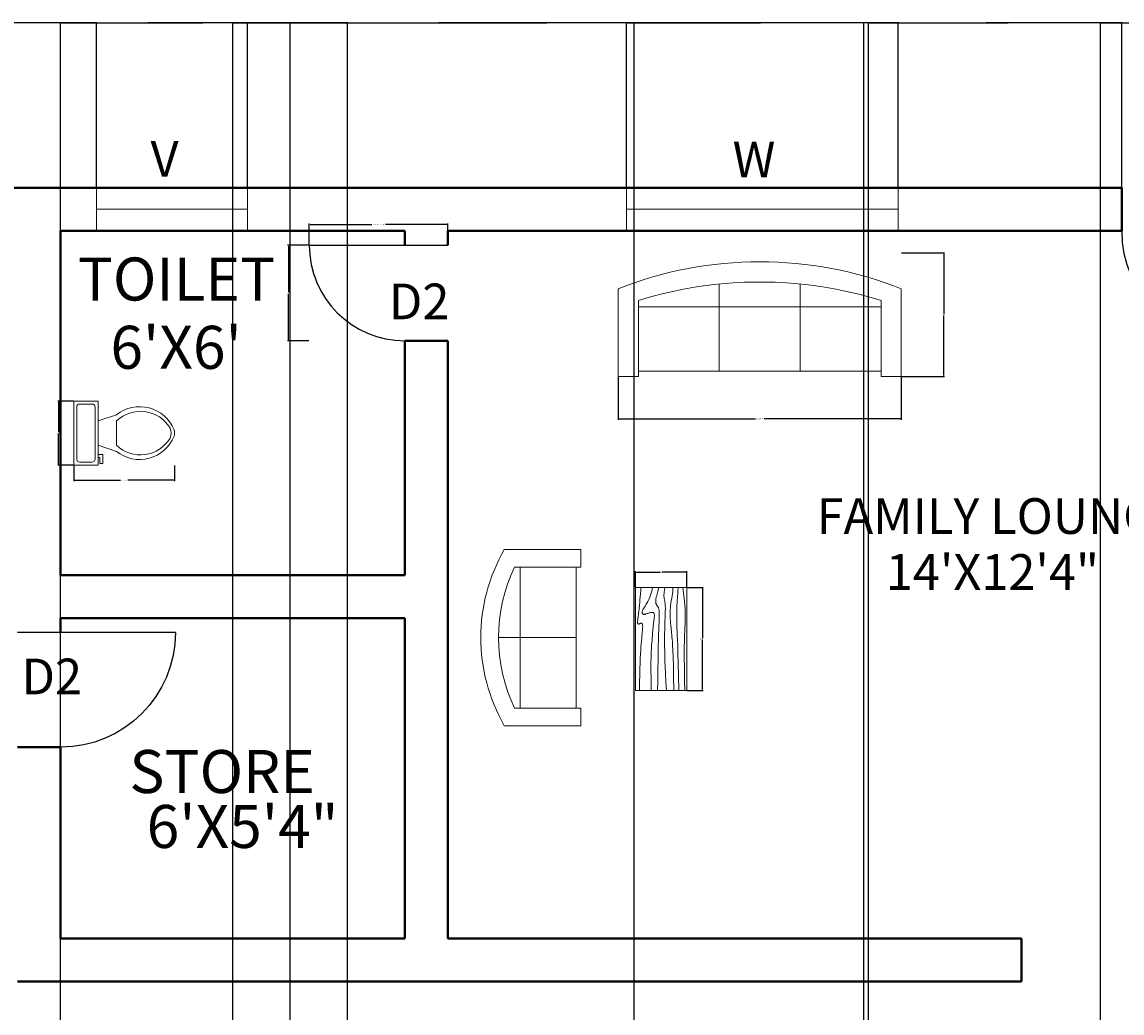
# Model space of a CAD drawing. Units: feet. Extents: x 2032 to 2763, y 1402 to 2145.
# Tile 5 of 6: x 2285 to 2515, y 1938 to 2145. Entities that reach past the tile are written whole.
import ezdxf

# ---------------------------------------------------------------- set-up
doc = ezdxf.new("R2010")
doc.units = ezdxf.units.FT
for name, color, linetype, lineweight in [('A-ANNO-DIMS', 2, 'Continuous', 18), ('A-ANNO-TEXT', 7, 'Continuous', 18), ('A-AREA-IDEN', 7, 'Continuous', 25), ('A-DOOR', 3, 'Continuous', 25), ('A-FLOR-FIXT', 8, 'Continuous', 18), ('A-FURN', 8, 'Continuous', 18), ('A-GLAZ', 4, 'Continuous', 18), ('A-WALL', 7, 'Continuous', 40)]:
    doc.layers.add(name, color=color, linetype=linetype, lineweight=lineweight)
doc.styles.get("Standard").update_dxf_attribs({"font": 'arial.ttf'})
doc.dimstyles.get("Standard").update_dxf_attribs({"dimtxt": 0.18, "dimasz": 0.18, "dimexe": 0.18, "dimexo": 0.0625, "dimgap": 0.09, "dimtad": 0, "dimtih": 1, "dimtoh": 1, "dimdec": 4, "dimzin": 0, "dimdsep": 46, "dimtxsty": 'Standard', "dimcen": 0.09, "dimadec": 0, "dimazin": 0, "dimtfac": 1, "dimtdec": 4, "dimtofl": 0, "dimtmove": 0, "dimatfit": 3, "dimfxl": 1, "dimtolj": 1, "dimtzin": 0, "dimarcsym": 0})

# ---------------------------------------------------------------- blocks, each defined once
blk = doc.blocks.new('Toilet - top')
for p, q in [((9.5, -6), (9.5, -2)), ((-10, -8.5), (-8, -8.5)), ((-10, -9.5), (-10, -8.5)), ((-7, -9.5), (-10, -9.5)), ((-8, -8.5), (-8, -8)), ((-7, -8), (-7, -9.5)), ((-4, -8), (-6, -14)), ((4, -8), (6, -14)), ((4, -14), (-4, -14))]:
    blk.add_line(p, q)
blk.add_lwpolyline([(10.5, -8), (10.5, 0), (-10.5, 0), (-10.5, -8)], close=True)
for points in [[(-9.5, -2), (-9.5, -6)], [(8.5, -1), (-8.5, -1)], [(-8.5, -7), (8.5, -7)]]:
    blk.add_lwpolyline(points)
for centre, radius, start, end in [((-8.62, -1.88), 0.884, 81.8699, 188.1301), ((8.62, -1.88), 0.884, 351.8699, 98.1301), ((-8.62, -6.12), 0.884, 171.8699, 278.1301), ((8.62, -6.12), 0.884, 261.8699, 8.1301), ((3.52, -21.58), 12.17, 141.4691, 247.9714), ((4.2, -21.82), 11.33, 136.3677, 238.9468), ((-3.52, -21.58), 12.17, 292.0284, 38.5307), ((-4.2, -21.82), 11.33, 301.053, 43.6321), ((0, -27.88), 4, 245.7318, 294.2682), ((0, -29), 4, 254.8605, 285.1395)]:
    blk.add_arc(centre, radius, start, end)
blk = doc.blocks.new('Sofa - Roundback 7 ft.')
for p, q in [((-12.00002, -32.4421), (-12.00003, -6.5971)), ((11.99997, -32.4421), (11.99998, -6.5971)), ((-36.000027, -34), (-36.000027, -11.4696)), ((35.99998, -34), (35.99998, -11.4696)), ((-35.999844, -13.3819), (35.9998, -13.3819)), ((-36.000027, -32.4421), (35.99998, -32.4421))]:
    blk.add_line(p, q)
for points in [[(-36.000027, -34), (-42.000027, -34), (-42.000027, -8)], [(41.99998, -8), (41.99998, -34), (35.99998, -34)]]:
    blk.add_lwpolyline(points)
for centre, radius, start, end in [((0, -114.25), 114.25, 68.43141, 111.5686), ((-0.00001, -127.1968), 121.1968, 72.72033, 107.2797)]:
    blk.add_arc(centre, radius, start, end)
blk = doc.blocks.new('Sofa - Roundback Loveseat 5 ft.')
for p, q in [((0, -32.44198), (0, -5.99998)), ((-24, -33.99998), (-24, -11.46958)), ((-23.9998, -13.38178), (23.99986, -13.38178)), ((24.00004, -33.99998), (24.00004, -11.46958)), ((-24, -32.44198), (24.00004, -32.44198))]:
    blk.add_line(p, q)
for points in [[(-24, -33.99998), (-30, -33.99998), (-30, -7.99998)], [(30.00004, -7.99998), (30.00004, -33.99998), (24.00004, -33.99998)]]:
    blk.add_lwpolyline(points)
for centre, radius, start, end in [((0, -60.24998), 60.24998, 60.13715, 119.8628), ((0, -61.38438), 55.38444, 64.32083, 115.6792)]:
    blk.add_arc(centre, radius, start, end)
blk = doc.blocks.new('Table - Rectangular Woodgrain 60 x 30 in.')
for p, q in [((0, 0), (0, -30)), ((60, 0), (0, 0)), ((60, -30), (60, 0)), ((0, -30), (60, -30))]:
    blk.add_line(p, q)
for points in [[(0, -2.4), (4.8155, -2.418), (9.0302, -2.4688), (12.709, -2.5477), (15.9167, -2.65), (18.7181, -2.7711), (21.1781, -2.9063), (23.3616, -3.0508), (25.3333, -3.2), (27.1477, -3.3495), (28.8172, -3.4958), (30.3437, -3.636), (31.7291, -3.7667), (32.9756, -3.8849), (34.0849, -3.9875), (35.059, -4.0714), (35.9, -4.1334), (36.6114, -4.1711), (37.2041, -4.1854), (37.6906, -4.1779), (38.0833, -4.15), (38.3948, -4.1034), (38.6375, -4.0396), (38.8239, -3.9602), (38.9666, -3.8667), (39.0764, -3.7608), (39.1573, -3.6448), (39.2116, -3.521), (39.2416, -3.3917), (39.2498, -3.2593), (39.2385, -3.1261), (39.21, -2.9944), (39.1666, -2.8667), (39.111, -2.7447), (39.0468, -2.6281), (38.978, -2.5163), (38.9083, -2.4083), (38.8418, -2.3035), (38.7823, -2.201), (38.7337, -2.1001), (38.7, -2), (38.6844, -1.9003), (38.6875, -1.8021), (38.7094, -1.707), (38.75, -1.6167), (38.8094, -1.5326), (38.8875, -1.4563), (38.9844, -1.3893), (39.1, -1.3333), (39.2351, -1.2896), (39.3937, -1.2583), (39.5804, -1.2396), (39.8, -1.2333), (40.057, -1.2396), (40.3562, -1.2583), (40.7023, -1.2896), (41.1, -1.3333), (41.5547, -1.3895), (42.0755, -1.4573), (42.6721, -1.5361), (43.3542, -1.625), (44.1316, -1.7233), (45.014, -1.8302), (46.0114, -1.9449), (47.1333, -2.0667), (48.3862, -2.1947), (49.7625, -2.3281), (51.2513, -2.4663), (52.8416, -2.6083), (54.5226, -2.7535), (56.2833, -2.9011), (58.1127, -3.0501), (60, -3.2)], [(0, -9.2), (6.5759, -9.0858), (11.9385, -9.0365), (16.2527, -9.0418), (19.6833, -9.0917), (22.3952, -9.1759), (24.5531, -9.2844), (26.322, -9.4069), (27.8666, -9.5333), (29.3241, -9.6553), (30.7203, -9.7719), (32.0532, -9.8837), (33.3208, -9.9917), (34.5213, -10.0965), (35.6526, -10.199), (36.7128, -10.2999), (37.7, -10.4), (38.6129, -10.4996), (39.4531, -10.5969), (40.223, -10.6895), (40.925, -10.775), (41.5613, -10.8512), (42.1344, -10.9156), (42.6465, -10.966), (43.1, -11), (43.4976, -11.0158), (43.8437, -11.0136), (44.143, -10.9942), (44.4, -10.9583), (44.6195, -10.9069), (44.8062, -10.8406), (44.9648, -10.7603), (45.1, -10.6667), (45.2155, -10.5598), (45.3114, -10.4365), (45.3871, -10.2929), (45.4416, -10.125), (45.4743, -9.929), (45.4844, -9.7011), (45.4709, -9.4371), (45.4333, -9.1333), (45.3716, -8.7883), (45.2896, -8.4104), (45.1919, -8.0107), (45.0833, -7.6), (44.9685, -7.1893), (44.8521, -6.7896), (44.7388, -6.4117), (44.6333, -6.0667), (44.54, -5.7628), (44.4614, -5.4979), (44.4001, -5.2675), (44.3583, -5.0667), (44.3384, -4.8909), (44.3427, -4.7354), (44.3736, -4.5956), (44.4333, -4.4667), (44.5236, -4.3453), (44.6427, -4.2333), (44.7884, -4.1339), (44.9583, -4.05), (45.1501, -3.9849), (45.3614, -3.9417), (45.59, -3.9234), (45.8333, -3.9333), (46.0915, -3.9749), (46.3734, -4.0531), (46.6906, -4.1736), (47.0542, -4.3417), (47.4756, -4.5629), (47.9661, -4.8427), (48.5372, -5.1866), (49.2, -5.6), (49.9676, -6.0844), (50.8594, -6.625), (51.8965, -7.2031), (53.1, -7.8), (54.491, -8.3969), (56.0906, -8.975), (57.9199, -9.5156), (60, -10)], [(0, -12.8), (5.1847, -12.9322), (9.6213, -13.0323), (13.3963, -13.1059), (16.5958, -13.1583), (19.3063, -13.1952), (21.614, -13.2219), (23.6054, -13.2439), (25.3666, -13.2667), (26.9728, -13.2947), (28.4531, -13.3281), (29.8256, -13.3663), (31.1083, -13.4083), (32.3191, -13.4535), (33.476, -13.501), (34.597, -13.5501), (35.7, -13.6), (36.7984, -13.6497), (37.8875, -13.6979), (38.9578, -13.743), (40, -13.7833), (41.0047, -13.8174), (41.9625, -13.8438), (42.864, -13.8607), (43.7, -13.8667), (44.4631, -13.8604), (45.1552, -13.8417), (45.7801, -13.8104), (46.3416, -13.7667), (46.8439, -13.7104), (47.2906, -13.6417), (47.6858, -13.5604), (48.0333, -13.4667), (48.3375, -13.3608), (48.6042, -13.2448), (48.8396, -13.121), (49.05, -12.9917), (49.2417, -12.8593), (49.4208, -12.7261), (49.5937, -12.5944), (49.7667, -12.4667), (49.9452, -12.3451), (50.1323, -12.2313), (50.3303, -12.1268), (50.5416, -12.0333), (50.7686, -11.9524), (51.0135, -11.8854), (51.2788, -11.8341), (51.5666, -11.8), (51.8785, -11.7843), (52.2116, -11.7865), (52.562, -11.8059), (52.926, -11.8417), (53.2998, -11.8931), (53.6795, -11.9594), (54.0614, -12.0397), (54.4416, -12.1333), (54.8223, -12.2401), (55.2293, -12.3625), (55.6942, -12.5037), (56.2489, -12.6667), (56.9251, -12.8547), (57.7545, -13.0708), (58.7689, -13.3182), (60, -13.6)], [(0, -18), (5.124, -17.7273), (9.6609, -17.5057), (13.6705, -17.3303), (17.2125, -17.1958), (20.3467, -17.0973), (23.1328, -17.0297), (25.6307, -16.9878), (27.9, -16.9667), (29.9928, -16.9617), (31.9302, -16.9703), (33.7254, -16.9907), (35.3917, -17.0208), (36.9423, -17.0588), (38.3906, -17.1026), (39.7499, -17.1503), (41.0333, -17.2), (42.2519, -17.2496), (43.4073, -17.2969), (44.4986, -17.3395), (45.525, -17.375), (46.4858, -17.4012), (47.3802, -17.4156), (48.2074, -17.416), (48.9667, -17.4), (49.6583, -17.3662), (50.2872, -17.3167), (50.8595, -17.2547), (51.3812, -17.1833), (51.8584, -17.1057), (52.2971, -17.025), (52.7034, -16.9443), (53.0833, -16.8667), (53.443, -16.7951), (53.789, -16.7313), (54.128, -16.6768), (54.4666, -16.6334), (54.8115, -16.6024), (55.1693, -16.5854), (55.5465, -16.5841), (55.95, -16.6), (56.3828, -16.6337), (56.8346, -16.6823), (57.2915, -16.7418), (57.7396, -16.8084), (58.165, -16.878), (58.5539, -16.9469), (58.8924, -17.0111), (59.1666, -17.0667), (59.3679, -17.1107), (59.5078, -17.1438), (59.6032, -17.1675), (59.6708, -17.1833), (59.7275, -17.193), (59.7901, -17.1979), (59.8753, -17.1998), (60, -17.2)], [(0, -22.4), (8.0098, -22.2501), (14.4094, -22.1011), (19.4168, -21.9535), (23.25, -21.8083), (26.1269, -21.6663), (28.2656, -21.5281), (29.884, -21.3947), (31.2, -21.2667), (32.3967, -21.1448), (33.5172, -21.0292), (34.5697, -20.9198), (35.5625, -20.8167), (36.5037, -20.7198), (37.4015, -20.6292), (38.2642, -20.5448), (39.1, -20.4667), (39.9164, -20.3951), (40.7187, -20.3313), (41.5117, -20.2768), (42.3, -20.2333), (43.0883, -20.2024), (43.8812, -20.1854), (44.6836, -20.1841), (45.5, -20.2), (46.3328, -20.234), (47.1747, -20.2844), (48.0163, -20.3488), (48.8479, -20.425), (49.66, -20.5106), (50.4429, -20.6031), (51.1872, -20.7004), (51.8833, -20.8), (52.5246, -20.8999), (53.1166, -20.9995), (53.6681, -21.0983), (54.1875, -21.1958), (54.6834, -21.2919), (55.1646, -21.3859), (55.6394, -21.4777), (56.1167, -21.5667), (56.6028, -21.6515), (57.0961, -21.7266), (57.5929, -21.7852), (58.0896, -21.8208), (58.5823, -21.8268), (59.0674, -21.7964), (59.5412, -21.723), (60, -21.6)], [(0, -25.2), (8.6355, -25.0504), (15.7026, -24.9031), (21.4049, -24.7606), (25.9458, -24.625), (29.529, -24.4988), (32.3578, -24.3844), (34.6359, -24.284), (36.5667, -24.2), (38.3213, -24.1341), (39.9417, -24.0854), (41.437, -24.0523), (42.8167, -24.0333), (44.0901, -24.0268), (45.2667, -24.0313), (46.3557, -24.0451), (47.3667, -24.0667), (48.309, -24.0947), (49.1928, -24.1287), (50.0284, -24.168), (50.826, -24.2125), (51.5959, -24.2617), (52.3483, -24.3151), (53.0935, -24.3725), (53.8417, -24.4334), (54.6009, -24.497), (55.3699, -24.561), (56.1454, -24.6226), (56.9239, -24.6792), (57.7021, -24.7279), (58.4764, -24.7662), (59.2435, -24.7911), (60, -24.8)], [(0, -28.8), (5.6867, -28.6681), (10.45, -28.5698), (14.407, -28.5012), (17.675, -28.4584), (20.3711, -28.4374), (22.6125, -28.4344), (24.5164, -28.4455), (26.2, -28.4667), (27.762, -28.4947), (29.2276, -28.5281), (30.6033, -28.5663), (31.8958, -28.6084), (33.1118, -28.6535), (34.2578, -28.7011), (35.3405, -28.7501), (36.3666, -28.8), (37.3443, -28.8497), (38.288, -28.8974), (39.2137, -28.9412), (40.1375, -28.9792), (41.0753, -29.0093), (42.0432, -29.0297), (43.0572, -29.0384), (44.1333, -29.0333), (45.2936, -29.0114), (46.5843, -28.9641), (48.0579, -28.8816), (49.7666, -28.7542), (51.7629, -28.5721), (54.0989, -28.3255), (56.8272, -28.0048), (60, -27.6)]]:
    blk.add_lwpolyline(points)
blk = doc.blocks.new('DOOR-SWING-24')
blk.add_line((33, 0), (0, 0))
blk.add_arc((9, 0), 24, 0, 90)
blk = doc.blocks.new('DOOR-SWING-20')
blk.add_line((0, 20), (29, 20))
blk.add_arc((20, 20), 20, 180, 270)
blk = doc.blocks.new('*D13')
at = {"layer": 'A-ANNO-DIMS', "color": 0, "lineweight": -2, "transparency": 16777216}
for p, q in [((2296.05, 2052.54), (2296.05, 2049.26)), ((2317.16, 2052.54), (2317.16, 2049.26)), ((2296.23, 2049.44), (2305.83, 2049.44)), ((2316.98, 2049.44), (2307.38, 2049.44))]:
    blk.add_line(p, q, dxfattribs=at)
at = {"layer": 'A-ANNO-DIMS', "color": 0, "transparency": 16777216}
for points in [[(2296.23, 2049.47), (2296.23, 2049.41), (2296.05, 2049.44)], [(2316.98, 2049.47), (2316.98, 2049.41), (2317.16, 2049.44)]]:
    blk.add_solid(points, dxfattribs=at)
at = {"layer": 'Defpoints', "color": 0, "transparency": 16777216}
for p in [(2296.05, 2052.6), (2317.16, 2052.6), (2296.05, 2049.44)]:
    blk.add_point(p, dxfattribs=at)
at = {"layer": 'A-ANNO-DIMS', "color": 0, "transparency": 16777216, "insert": (2306.61, 2049.44), "char_height": 0.18, "attachment_point": 5}
blk.add_mtext('\\A1;WC 21 TYP.', dxfattribs=at)
blk = doc.blocks.new('*D14')
at = {"layer": 'A-ANNO-DIMS', "color": 0, "lineweight": -2, "transparency": 16777216}
for p, q in [((2295.99, 2066.02), (2292.7, 2066.02)), ((2292.88, 2065.84), (2292.88, 2059.49)), ((2292.88, 2052.78), (2292.88, 2059.13)), ((2295.99, 2052.6), (2292.7, 2052.6))]:
    blk.add_line(p, q, dxfattribs=at)
at = {"layer": 'A-ANNO-DIMS', "color": 0, "transparency": 16777216}
for points in [[(2292.85, 2065.84), (2292.91, 2065.84), (2292.88, 2066.02)], [(2292.85, 2052.78), (2292.91, 2052.78), (2292.88, 2052.6)]]:
    blk.add_solid(points, dxfattribs=at)
at = {"layer": 'Defpoints', "color": 0, "transparency": 16777216}
for p in [(2292.88, 2066.02), (2296.05, 2066.02), (2296.05, 2052.6)]:
    blk.add_point(p, dxfattribs=at)
at = {"layer": 'A-ANNO-DIMS', "color": 0, "transparency": 16777216, "insert": (2292.88, 2059.31), "char_height": 0.18, "attachment_point": 5}
blk.add_mtext('\\A1;13 TYP.', dxfattribs=at)
blk = doc.blocks.new('*D17')
at = {"layer": 'A-ANNO-DIMS', "color": 0, "lineweight": -2, "transparency": 16777216}
for p, q in [((2409.94, 2071.12), (2409.94, 2062.12)), ((2469.15, 2071.12), (2469.15, 2062.12)), ((2410.12, 2062.3), (2438.64, 2062.3)), ((2468.97, 2062.3), (2440.45, 2062.3))]:
    blk.add_line(p, q, dxfattribs=at)
at = {"layer": 'A-ANNO-DIMS', "color": 0, "transparency": 16777216}
for points in [[(2410.12, 2062.33), (2410.12, 2062.27), (2409.94, 2062.3)], [(2468.97, 2062.33), (2468.97, 2062.27), (2469.15, 2062.3)]]:
    blk.add_solid(points, dxfattribs=at)
at = {"layer": 'Defpoints', "color": 0, "transparency": 16777216}
for p in [(2409.94, 2071.18), (2469.15, 2071.18), (2469.15, 2062.3)]:
    blk.add_point(p, dxfattribs=at)
at = {"layer": 'A-ANNO-DIMS', "color": 0, "transparency": 16777216, "insert": (2439.54, 2062.3), "char_height": 0.18, "attachment_point": 5}
blk.add_mtext('\\A1;SOFA 59 TYP.', dxfattribs=at)
blk = doc.blocks.new('*D18')
at = {"layer": 'A-ANNO-DIMS', "color": 0, "lineweight": -2, "transparency": 16777216}
for p, q in [((2469.21, 2097.02), (2478.21, 2097.02)), ((2478.03, 2096.84), (2478.03, 2084.28)), ((2478.03, 2071.36), (2478.03, 2083.92)), ((2469.21, 2071.18), (2478.21, 2071.18))]:
    blk.add_line(p, q, dxfattribs=at)
at = {"layer": 'A-ANNO-DIMS', "color": 0, "transparency": 16777216}
for points in [[(2478, 2096.84), (2478.06, 2096.84), (2478.03, 2097.02)], [(2478, 2071.36), (2478.06, 2071.36), (2478.03, 2071.18)]]:
    blk.add_solid(points, dxfattribs=at)
at = {"layer": 'Defpoints', "color": 0, "transparency": 16777216}
for p in [(2469.15, 2097.02), (2478.03, 2097.02), (2469.15, 2071.18)]:
    blk.add_point(p, dxfattribs=at)
at = {"layer": 'A-ANNO-DIMS', "color": 0, "transparency": 16777216, "insert": (2478.03, 2084.1), "char_height": 0.18, "attachment_point": 5}
blk.add_mtext('\\A1;26 TYP.', dxfattribs=at)
blk = doc.blocks.new('*D21')
at = {"layer": 'A-ANNO-DIMS', "color": 0, "lineweight": -2, "transparency": 16777216}
for p, q in [((2424.38, 2027.01), (2427.72, 2027.01)), ((2427.54, 2026.83), (2427.54, 2016.42)), ((2427.54, 2005.66), (2427.54, 2016.06)), ((2424.38, 2005.48), (2427.72, 2005.48))]:
    blk.add_line(p, q, dxfattribs=at)
at = {"layer": 'A-ANNO-DIMS', "color": 0, "transparency": 16777216}
for points in [[(2427.51, 2026.83), (2427.57, 2026.83), (2427.54, 2027.01)], [(2427.51, 2005.66), (2427.57, 2005.66), (2427.54, 2005.48)]]:
    blk.add_solid(points, dxfattribs=at)
at = {"layer": 'Defpoints', "color": 0, "transparency": 16777216}
for p in [(2424.31, 2027.01), (2427.54, 2027.01), (2424.31, 2005.48)]:
    blk.add_point(p, dxfattribs=at)
at = {"layer": 'A-ANNO-DIMS', "color": 0, "transparency": 16777216, "insert": (2427.54, 2016.24), "char_height": 0.18, "attachment_point": 5}
blk.add_mtext('\\A1;TABLE 22', dxfattribs=at)
blk = doc.blocks.new('*D22')
at = {"layer": 'A-ANNO-DIMS', "color": 0, "lineweight": -2, "transparency": 16777216}
for p, q in [((2413.55, 2027.07), (2413.55, 2030.41)), ((2413.73, 2030.23), (2418.74, 2030.23)), ((2424.13, 2030.23), (2419.13, 2030.23)), ((2424.31, 2027.07), (2424.31, 2030.41))]:
    blk.add_line(p, q, dxfattribs=at)
at = {"layer": 'A-ANNO-DIMS', "color": 0, "transparency": 16777216}
for points in [[(2413.73, 2030.26), (2413.73, 2030.2), (2413.55, 2030.23)], [(2424.13, 2030.26), (2424.13, 2030.2), (2424.31, 2030.23)]]:
    blk.add_solid(points, dxfattribs=at)
at = {"layer": 'Defpoints', "color": 0, "transparency": 16777216}
for p in [(2413.55, 2030.23), (2413.55, 2027.01), (2424.31, 2027.01)]:
    blk.add_point(p, dxfattribs=at)
at = {"layer": 'A-ANNO-DIMS', "color": 0, "transparency": 16777216, "insert": (2418.93, 2030.23), "char_height": 0.18, "attachment_point": 5}
blk.add_mtext('\\A1;11', dxfattribs=at)
blk = doc.blocks.new('*D25')
at = {"layer": 'A-ANNO-DIMS', "color": 0, "lineweight": -2, "transparency": 16777216}
for p, q in [((2345.31, 2098.68), (2345.31, 2103.14)), ((2345.49, 2102.96), (2358.4, 2102.96)), ((2374.13, 2102.96), (2361.23, 2102.96)), ((2374.31, 2098.68), (2374.31, 2103.14))]:
    blk.add_line(p, q, dxfattribs=at)
at = {"layer": 'A-ANNO-DIMS', "color": 0, "transparency": 16777216}
for points in [[(2345.49, 2102.99), (2345.49, 2102.93), (2345.31, 2102.96)], [(2374.13, 2102.99), (2374.13, 2102.93), (2374.31, 2102.96)]]:
    blk.add_solid(points, dxfattribs=at)
at = {"layer": 'Defpoints', "color": 0, "transparency": 16777216}
for p in [(2374.31, 2102.96), (2345.31, 2098.61), (2374.31, 2098.61)]:
    blk.add_point(p, dxfattribs=at)
at = {"layer": 'A-ANNO-DIMS', "color": 0, "transparency": 16777216, "insert": (2359.81, 2102.96), "char_height": 0.18, "attachment_point": 5}
blk.add_mtext('\\A1;TOILET DOOR 29 TYP.', dxfattribs=at)
blk = doc.blocks.new('*D26')
at = {"layer": 'A-ANNO-DIMS', "color": 0, "lineweight": -2, "transparency": 16777216}
for p, q in [((2345.25, 2098.61), (2340.78, 2098.61)), ((2340.96, 2098.43), (2340.96, 2088.79)), ((2340.96, 2078.79), (2340.96, 2088.43)), ((2345.25, 2078.61), (2340.78, 2078.61))]:
    blk.add_line(p, q, dxfattribs=at)
at = {"layer": 'A-ANNO-DIMS', "color": 0, "transparency": 16777216}
for points in [[(2340.93, 2098.43), (2340.99, 2098.43), (2340.96, 2098.61)], [(2340.93, 2078.79), (2340.99, 2078.79), (2340.96, 2078.61)]]:
    blk.add_solid(points, dxfattribs=at)
at = {"layer": 'Defpoints', "color": 0, "transparency": 16777216}
for p in [(2340.96, 2098.61), (2345.31, 2098.61), (2345.31, 2078.61)]:
    blk.add_point(p, dxfattribs=at)
at = {"layer": 'A-ANNO-DIMS', "color": 0, "transparency": 16777216, "insert": (2340.96, 2088.61), "char_height": 0.18, "attachment_point": 5}
blk.add_mtext('\\A1;20 TYP.', dxfattribs=at)
blk = doc.blocks.new('*D38')
at = {"layer": 'A-ANNO-DIMS', "color": 0, "lineweight": -2, "transparency": 16777216}
for p, q in [((2239.45, 2110.68), (2239.45, 2145.29)), ((2239.63, 2145.11), (2269.73, 2145.11)), ((2300.62, 2145.11), (2270.52, 2145.11)), ((2300.8, 2110.68), (2300.8, 2145.29))]:
    blk.add_line(p, q, dxfattribs=at)
at = {"layer": 'A-ANNO-DIMS', "color": 0, "transparency": 16777216}
for points in [[(2239.63, 2145.14), (2239.63, 2145.08), (2239.45, 2145.11)], [(2300.62, 2145.14), (2300.62, 2145.08), (2300.8, 2145.11)]]:
    blk.add_solid(points, dxfattribs=at)
at = {"layer": 'Defpoints', "color": 0, "transparency": 16777216}
for p in [(2300.8, 2145.11), (2239.45, 2110.61), (2300.8, 2110.61)]:
    blk.add_point(p, dxfattribs=at)
at = {"layer": 'A-ANNO-DIMS', "color": 0, "transparency": 16777216, "insert": (2270.12, 2145.11), "char_height": 0.18, "attachment_point": 5}
blk.add_mtext('\\A1;61.36', dxfattribs=at)
blk = doc.blocks.new('*D39')
at = {"layer": 'A-ANNO-DIMS', "color": 0, "lineweight": -2, "transparency": 16777216}
for p, q in [((2300.8, 2110.68), (2300.8, 2145.29)), ((2300.98, 2145.11), (2316.19, 2145.11)), ((2332.19, 2145.11), (2316.98, 2145.11)), ((2332.37, 2110.68), (2332.37, 2145.29))]:
    blk.add_line(p, q, dxfattribs=at)
at = {"layer": 'A-ANNO-DIMS', "color": 0, "transparency": 16777216}
for points in [[(2300.98, 2145.14), (2300.98, 2145.08), (2300.8, 2145.11)], [(2332.19, 2145.14), (2332.19, 2145.08), (2332.37, 2145.11)]]:
    blk.add_solid(points, dxfattribs=at)
at = {"layer": 'Defpoints', "color": 0, "transparency": 16777216}
for p in [(2332.37, 2145.11), (2300.8, 2110.61), (2332.37, 2110.61)]:
    blk.add_point(p, dxfattribs=at)
at = {"layer": 'A-ANNO-DIMS', "color": 0, "transparency": 16777216, "insert": (2316.59, 2145.11), "char_height": 0.18, "attachment_point": 5}
blk.add_mtext('\\A1;31.57', dxfattribs=at)
blk = doc.blocks.new('*D40')
at = {"layer": 'A-ANNO-DIMS', "color": 0, "lineweight": -2, "transparency": 16777216}
for p, q in [((2332.37, 2110.68), (2332.37, 2145.29)), ((2332.55, 2145.11), (2371.7, 2145.11)), ((2411.49, 2145.11), (2372.35, 2145.11)), ((2411.67, 2110.68), (2411.67, 2145.29))]:
    blk.add_line(p, q, dxfattribs=at)
at = {"layer": 'A-ANNO-DIMS', "color": 0, "transparency": 16777216}
for points in [[(2332.55, 2145.14), (2332.55, 2145.08), (2332.37, 2145.11)], [(2411.49, 2145.14), (2411.49, 2145.08), (2411.67, 2145.11)]]:
    blk.add_solid(points, dxfattribs=at)
at = {"layer": 'Defpoints', "color": 0, "transparency": 16777216}
for p in [(2411.67, 2145.11), (2332.37, 2110.61), (2411.67, 2110.61)]:
    blk.add_point(p, dxfattribs=at)
at = {"layer": 'A-ANNO-DIMS', "color": 0, "transparency": 16777216, "insert": (2372.02, 2145.11), "char_height": 0.18, "attachment_point": 5}
blk.add_mtext('\\A1;79.3', dxfattribs=at)
blk = doc.blocks.new('*D41')
at = {"layer": 'A-ANNO-DIMS', "color": 0, "lineweight": -2, "transparency": 16777216}
for p, q in [((2411.67, 2110.68), (2411.67, 2145.29)), ((2411.85, 2145.11), (2439.7, 2145.11)), ((2468.34, 2145.11), (2440.49, 2145.11)), ((2468.52, 2110.68), (2468.52, 2145.29))]:
    blk.add_line(p, q, dxfattribs=at)
at = {"layer": 'A-ANNO-DIMS', "color": 0, "transparency": 16777216}
for points in [[(2411.85, 2145.14), (2411.85, 2145.08), (2411.67, 2145.11)], [(2468.34, 2145.14), (2468.34, 2145.08), (2468.52, 2145.11)]]:
    blk.add_solid(points, dxfattribs=at)
at = {"layer": 'Defpoints', "color": 0, "transparency": 16777216}
for p in [(2468.52, 2145.11), (2411.67, 2110.61), (2468.52, 2110.61)]:
    blk.add_point(p, dxfattribs=at)
at = {"layer": 'A-ANNO-DIMS', "color": 0, "transparency": 16777216, "insert": (2440.1, 2145.11), "char_height": 0.18, "attachment_point": 5}
blk.add_mtext('\\A1;56.85', dxfattribs=at)
blk = doc.blocks.new('*D42')
at = {"layer": 'A-ANNO-DIMS', "color": 0, "lineweight": -2, "transparency": 16777216}
for p, q in [((2468.52, 2110.68), (2468.52, 2145.29)), ((2468.7, 2145.11), (2491.52, 2145.11)), ((2515.13, 2145.11), (2492.32, 2145.11)), ((2515.31, 2110.68), (2515.31, 2145.29))]:
    blk.add_line(p, q, dxfattribs=at)
at = {"layer": 'A-ANNO-DIMS', "color": 0, "transparency": 16777216}
for points in [[(2468.7, 2145.14), (2468.7, 2145.08), (2468.52, 2145.11)], [(2515.13, 2145.14), (2515.13, 2145.08), (2515.31, 2145.11)]]:
    blk.add_solid(points, dxfattribs=at)
at = {"layer": 'Defpoints', "color": 0, "transparency": 16777216}
for p in [(2515.31, 2145.11), (2468.52, 2110.61), (2515.31, 2110.61)]:
    blk.add_point(p, dxfattribs=at)
at = {"layer": 'A-ANNO-DIMS', "color": 0, "transparency": 16777216, "insert": (2491.92, 2145.11), "char_height": 0.18, "attachment_point": 5}
blk.add_mtext('\\A1;46.79', dxfattribs=at)
blk = doc.blocks.new('*D43')
at = {"layer": 'A-ANNO-DIMS', "color": 0, "lineweight": -2, "transparency": 16777216}
for p, q in [((2515.31, 2110.68), (2515.31, 2145.29)), ((2515.49, 2145.11), (2527.09, 2145.11)), ((2539.13, 2145.11), (2527.53, 2145.11)), ((2539.31, 2110.68), (2539.31, 2145.29))]:
    blk.add_line(p, q, dxfattribs=at)
at = {"layer": 'A-ANNO-DIMS', "color": 0, "transparency": 16777216}
for points in [[(2515.49, 2145.14), (2515.49, 2145.08), (2515.31, 2145.11)], [(2539.13, 2145.14), (2539.13, 2145.08), (2539.31, 2145.11)]]:
    blk.add_solid(points, dxfattribs=at)
at = {"layer": 'Defpoints', "color": 0, "transparency": 16777216}
for p in [(2539.31, 2145.11), (2515.31, 2110.61), (2539.31, 2110.61)]:
    blk.add_point(p, dxfattribs=at)
at = {"layer": 'A-ANNO-DIMS', "color": 0, "transparency": 16777216, "insert": (2527.31, 2145.11), "char_height": 0.18, "attachment_point": 5}
blk.add_mtext('\\A1;24', dxfattribs=at)
blk = doc.blocks.new('*D67')
at = {"layer": 'A-ANNO-DIMS', "color": 0, "lineweight": -2, "transparency": 16777216}
for p, q in [((2329.31, 1594.68), (2329.31, 2145.29)), ((2329.49, 2145.11), (2395.03, 2145.11)), ((2461.13, 2145.11), (2395.59, 2145.11)), ((2461.31, 1594.68), (2461.31, 2145.29))]:
    blk.add_line(p, q, dxfattribs=at)
at = {"layer": 'A-ANNO-DIMS', "color": 0, "transparency": 16777216}
for points in [[(2329.49, 2145.14), (2329.49, 2145.08), (2329.31, 2145.11)], [(2461.13, 2145.14), (2461.13, 2145.08), (2461.31, 2145.11)]]:
    blk.add_solid(points, dxfattribs=at)
at = {"layer": 'Defpoints', "color": 0, "transparency": 16777216}
for p in [(2461.31, 2145.11), (2329.31, 1594.61), (2461.31, 1594.61)]:
    blk.add_point(p, dxfattribs=at)
at = {"layer": 'A-ANNO-DIMS', "color": 0, "transparency": 16777216, "insert": (2395.31, 2145.11), "char_height": 0.18, "attachment_point": 5}
blk.add_mtext('\\A1;132', dxfattribs=at)
blk = doc.blocks.new('*D69')
at = {"layer": 'A-ANNO-DIMS', "color": 0, "lineweight": -2, "transparency": 16777216}
for p, q in [((2341.31, 1505.68), (2341.31, 2145.29)), ((2341.49, 2145.11), (2347.1, 2145.11)), ((2353.13, 2145.11), (2347.52, 2145.11)), ((2353.31, 1505.68), (2353.31, 2145.29))]:
    blk.add_line(p, q, dxfattribs=at)
at = {"layer": 'A-ANNO-DIMS', "color": 0, "transparency": 16777216}
for points in [[(2341.49, 2145.14), (2341.49, 2145.08), (2341.31, 2145.11)], [(2353.13, 2145.14), (2353.13, 2145.08), (2353.31, 2145.11)]]:
    blk.add_solid(points, dxfattribs=at)
at = {"layer": 'Defpoints', "color": 0, "transparency": 16777216}
for p in [(2353.31, 2145.11), (2341.31, 1505.61), (2353.31, 1505.61)]:
    blk.add_point(p, dxfattribs=at)
at = {"layer": 'A-ANNO-DIMS', "color": 0, "transparency": 16777216, "insert": (2347.31, 2145.11), "char_height": 0.18, "attachment_point": 5}
blk.add_mtext('\\A1;12', dxfattribs=at)
blk = doc.blocks.new('*D72')
at = {"layer": 'A-ANNO-DIMS', "color": 0, "lineweight": -2, "transparency": 16777216}
for p, q in [((2293.31, 1505.68), (2293.31, 2145.29)), ((2293.49, 2145.11), (2311.09, 2145.11)), ((2329.13, 2145.11), (2311.53, 2145.11)), ((2329.31, 1501.18), (2329.31, 2145.29))]:
    blk.add_line(p, q, dxfattribs=at)
at = {"layer": 'A-ANNO-DIMS', "color": 0, "transparency": 16777216}
for points in [[(2293.49, 2145.14), (2293.49, 2145.08), (2293.31, 2145.11)], [(2329.13, 2145.14), (2329.13, 2145.08), (2329.31, 2145.11)]]:
    blk.add_solid(points, dxfattribs=at)
at = {"layer": 'Defpoints', "color": 0, "transparency": 16777216}
for p in [(2329.31, 2145.11), (2293.31, 1505.61), (2329.31, 1501.11)]:
    blk.add_point(p, dxfattribs=at)
at = {"layer": 'A-ANNO-DIMS', "color": 0, "transparency": 16777216, "insert": (2311.31, 2145.11), "char_height": 0.18, "attachment_point": 5}
blk.add_mtext('\\A1;36', dxfattribs=at)
blk = doc.blocks.new('*D73')
at = {"layer": 'A-ANNO-DIMS', "color": 0, "lineweight": -2, "transparency": 16777216}
for p, q in [((2462.31, 1775.68), (2462.31, 2145.29)), ((2462.49, 2145.11), (2486.24, 2145.11)), ((2510.63, 2145.11), (2486.89, 2145.11)), ((2510.81, 1775.68), (2510.81, 2145.29))]:
    blk.add_line(p, q, dxfattribs=at)
at = {"layer": 'A-ANNO-DIMS', "color": 0, "transparency": 16777216}
for points in [[(2462.49, 2145.14), (2462.49, 2145.08), (2462.31, 2145.11)], [(2510.63, 2145.14), (2510.63, 2145.08), (2510.81, 2145.11)]]:
    blk.add_solid(points, dxfattribs=at)
at = {"layer": 'Defpoints', "color": 0, "transparency": 16777216}
for p in [(2510.81, 2145.11), (2462.31, 1775.61), (2510.81, 1775.61)]:
    blk.add_point(p, dxfattribs=at)
at = {"layer": 'A-ANNO-DIMS', "color": 0, "transparency": 16777216, "insert": (2486.56, 2145.11), "char_height": 0.18, "attachment_point": 5}
blk.add_mtext('\\A1;48.5', dxfattribs=at)
blk = doc.blocks.new('*D74')
at = {"layer": 'A-ANNO-DIMS', "color": 0, "lineweight": -2, "transparency": 16777216}
for p, q in [((2510.81, 1775.68), (2510.81, 2145.29)), ((2510.99, 2145.11), (2534.59, 2145.11)), ((2558.63, 2145.11), (2535.04, 2145.11)), ((2558.81, 1775.68), (2558.81, 2145.29))]:
    blk.add_line(p, q, dxfattribs=at)
at = {"layer": 'A-ANNO-DIMS', "color": 0, "transparency": 16777216}
for points in [[(2510.99, 2145.14), (2510.99, 2145.08), (2510.81, 2145.11)], [(2558.63, 2145.14), (2558.63, 2145.08), (2558.81, 2145.11)]]:
    blk.add_solid(points, dxfattribs=at)
at = {"layer": 'Defpoints', "color": 0, "transparency": 16777216}
for p in [(2558.81, 2145.11), (2510.81, 1775.61), (2558.81, 1775.61)]:
    blk.add_point(p, dxfattribs=at)
at = {"layer": 'A-ANNO-DIMS', "color": 0, "transparency": 16777216, "insert": (2534.81, 2145.11), "char_height": 0.18, "attachment_point": 5}
blk.add_mtext('\\A1;48', dxfattribs=at)
blk = doc.blocks.new('*D79')
at = {"layer": 'A-ANNO-DIMS', "color": 0, "lineweight": -2, "transparency": 16777216}
for p, q in [((2353.31, 1603.68), (2353.31, 2145.29)), ((2353.49, 2145.11), (2383.09, 2145.11)), ((2413.13, 2145.11), (2383.53, 2145.11)), ((2413.31, 1603.68), (2413.31, 2145.29))]:
    blk.add_line(p, q, dxfattribs=at)
at = {"layer": 'A-ANNO-DIMS', "color": 0, "transparency": 16777216}
for points in [[(2353.49, 2145.14), (2353.49, 2145.08), (2353.31, 2145.11)], [(2413.13, 2145.14), (2413.13, 2145.08), (2413.31, 2145.11)]]:
    blk.add_solid(points, dxfattribs=at)
at = {"layer": 'Defpoints', "color": 0, "transparency": 16777216}
for p in [(2413.31, 2145.11), (2353.31, 1603.61), (2413.31, 1603.61)]:
    blk.add_point(p, dxfattribs=at)
at = {"layer": 'A-ANNO-DIMS', "color": 0, "transparency": 16777216, "insert": (2383.31, 2145.11), "char_height": 0.18, "attachment_point": 5}
blk.add_mtext('\\A1;60', dxfattribs=at)
blk = doc.blocks.new('*D81')
at = {"layer": 'A-ANNO-DIMS', "color": 0, "lineweight": -2, "transparency": 16777216}
for p, q in [((2293.31, 1603.68), (2293.31, 2145.29)), ((2293.49, 2145.11), (2323.09, 2145.11)), ((2353.13, 2145.11), (2323.53, 2145.11)), ((2353.31, 1603.68), (2353.31, 2145.29))]:
    blk.add_line(p, q, dxfattribs=at)
at = {"layer": 'A-ANNO-DIMS', "color": 0, "transparency": 16777216}
for points in [[(2293.49, 2145.14), (2293.49, 2145.08), (2293.31, 2145.11)], [(2353.13, 2145.14), (2353.13, 2145.08), (2353.31, 2145.11)]]:
    blk.add_solid(points, dxfattribs=at)
at = {"layer": 'Defpoints', "color": 0, "transparency": 16777216}
for p in [(2353.31, 2145.11), (2293.31, 1603.61), (2353.31, 1603.61)]:
    blk.add_point(p, dxfattribs=at)
at = {"layer": 'A-ANNO-DIMS', "color": 0, "transparency": 16777216, "insert": (2323.31, 2145.11), "char_height": 0.18, "attachment_point": 5}
blk.add_mtext('\\A1;60', dxfattribs=at)

msp = doc.modelspace()

# ---------------------------------------------------------------- linework, layer by layer
at = {"layer": 'A-GLAZ'}
for p, q in [((2300.8003, 2110.6131), (2300.8003, 2101.6131)), ((2332.3721, 2110.6131), (2332.3721, 2101.6131)), ((2411.6726, 2110.6131), (2411.6726, 2101.6131)), ((2468.5217, 2110.6131), (2468.5217, 2101.6131)), ((2300.8003, 2106.1131), (2332.3721, 2106.1131)), ((2411.6726, 2106.1131), (2468.5217, 2106.1131))]:
    msp.add_line(p, q, dxfattribs=at)
at = {"layer": 'A-WALL'}
for p, q in [((2127.3136, 2110.6131), (2515.3136, 2110.6131)), ((2127.3136, 2110.6131), (2515.3136, 2110.6131)), ((2293.3136, 2110.6131), (2365.3136, 2110.6131)), ((2515.3136, 2110.6131), (2515.3136, 2101.6131)), ((2293.3136, 2101.6131), (2293.3136, 2029.6131)), ((2293.3136, 2101.6131), (2365.3136, 2101.6131)), ((2365.3136, 2101.6131), (2365.3136, 2098.6131)), ((2374.3136, 2101.6131), (2374.3136, 2098.6131)), ((2374.3136, 2101.6131), (2515.3136, 2101.6131)), ((2365.3136, 2078.6131), (2374.3136, 2078.6131)), ((2365.3136, 2078.6131), (2365.3136, 2029.6131)), ((2374.3136, 2078.6131), (2374.3136, 1953.6131)), ((2365.3136, 2029.6131), (2293.3136, 2029.6131)), ((2365.3136, 2020.6131), (2293.3136, 2020.6131)), ((2293.3136, 2020.6131), (2293.3136, 2017.6131)), ((2365.3136, 2020.6131), (2365.3136, 1953.6131)), ((2374.3136, 2020.6131), (2374.3136, 1953.6131)), ((2293.3136, 1993.6131), (2284.3136, 1993.6131)), ((2293.3136, 1993.6131), (2293.3136, 1953.6131)), ((2293.3136, 1953.6131), (2365.3136, 1953.6131)), ((2374.3136, 1953.6131), (2494.3136, 1953.6131)), ((2494.3136, 1953.6131), (2494.3136, 1944.6131)), ((2494.3136, 1944.6131), (2284.3136, 1944.6131)), ((2293.3136, 1944.6131), (2365.3136, 1944.6131)), ((2374.3136, 1944.6131), (2494.3136, 1944.6131))]:
    msp.add_line(p, q, dxfattribs=at)

# ---------------------------------------------------------------- block references
at = {"layer": 'A-DOOR', "extrusion": (0, 0, -1), "zscale": -1}
for p, rotation in [((-2539.3137, 2110.6127), 269.9999999999995), ((-2284.314, 2017.6131), 180)]:
    msp.add_blockref('DOOR-SWING-24', p, dxfattribs=dict(at, rotation=rotation))
at = {"layer": 'A-DOOR'}
msp.add_blockref('DOOR-SWING-20', (2345.314, 2078.613), dxfattribs=at)
at = {"layer": 'A-FLOR-FIXT', "xscale": 0.6388725113463674, "yscale": 0.6388725113463674, "zscale": 0.6388725113463674, "rotation": 90}
msp.add_blockref('Toilet - top', (2296.0507, 2059.3129), dxfattribs=at)
at = {"layer": 'A-FURN', "xscale": 0.7048316965902599, "yscale": 0.7048316965902599, "zscale": 0.7048316965902599}
msp.add_blockref('Sofa - Roundback 7 ft.', (2439.5432, 2095.1421), dxfattribs=at)
at = {"layer": 'A-FURN', "rotation": 90}
for name, p, xscale, yscale, zscale in [('Sofa - Roundback Loveseat 5 ft.', (2381.2027, 2016.553), 0.6145312403324517, 0.6145312403324517, 0.6145312403324517), ('Table - Rectangular Woodgrain 60 x 30 in.', (2413.5534, 2005.4826), 0.3587083407969354, 0.3587083407969354, 0.3587083407969354)]:
    msp.add_blockref(name, p, dxfattribs=dict(at, xscale=xscale, yscale=yscale, zscale=zscale))

# ---------------------------------------------------------------- texts
at = {"layer": 'A-ANNO-TEXT'}
for s, height, p in [('V', 7.4682, (2312.1249, 2112.9235)), ('W', 7.4682, (2433.8674, 2112.8028)), ('D2', 7.46821, (2361.9684, 2083.1151)), ('D2', 7.46821, (2285.1246, 2004.6735))]:
    msp.add_text(s, height=height, dxfattribs=at).set_placement(p)
at = {"layer": 'A-AREA-IDEN'}
for s, height, p in [('TOILET', 8.99902, (2296.885, 2087.0355)), ("6'X6'", 8.99902, (2303.7312, 2072.7594)), ('FAMILY LOUNGE', 7.468214, (2451.4477, 2038.2315)), ('14\'X12\'4"', 7.46821, (2465.9077, 2026.5293)), ('STORE', 8.99902, (2307.7098, 1984.0294)), ('6\'X5\'4"', 8.99902, (2311.3135, 1972.5411))]:
    msp.add_text(s, height=height, dxfattribs=at).set_placement(p)

# ---------------------------------------------------------------- dimensions: what is measured, and where the dimension line sits
at = {"layer": 'A-ANNO-DIMS'}
for base, p1, p2, override, picture, middle in [((2300.80031, 2145.11307), (2239.44528, 2110.61307), (2300.80031, 2110.61307), {"dimdec": 2, "dimlfac": 1, "dimrnd": 0, "dimzin": 0, "dimdsep": 46, "dimlunit": 2}, '*D38', (2270.12279, 2145.11307)), ((2329.3136, 2145.1131), (2293.3136, 1505.6131), (2329.3136, 1501.1131), {"dimdec": 0, "dimlfac": 1, "dimrnd": 0, "dimzin": 0, "dimdsep": 46, "dimlunit": 2}, '*D72', (2311.3136, 2145.1131)), ((2353.3136, 2145.1131), (2293.3136, 1603.6131), (2353.3136, 1603.6131), {"dimdec": 0, "dimlfac": 1, "dimrnd": 0, "dimzin": 0, "dimdsep": 46, "dimlunit": 2}, '*D81', (2323.3136, 2145.1131)), ((2332.3721, 2145.1131), (2300.8003, 2110.6131), (2332.3721, 2110.6131), {"dimdec": 2, "dimlfac": 1, "dimrnd": 0, "dimzin": 0, "dimdsep": 46, "dimlunit": 2}, '*D39', (2316.5862, 2145.1131)), ((2461.3136, 2145.1131), (2329.3136, 1594.6131), (2461.3136, 1594.6131), {"dimdec": 0, "dimlfac": 1, "dimrnd": 0, "dimzin": 0, "dimdsep": 46, "dimlunit": 2}, '*D67', (2395.3136, 2145.1131)), ((2411.6726, 2145.1131), (2332.3721, 2110.6131), (2411.6726, 2110.6131), {"dimdec": 1, "dimlfac": 1, "dimrnd": 0, "dimzin": 0, "dimdsep": 46, "dimlunit": 2}, '*D40', (2372.0223, 2145.1131)), ((2353.3136, 2145.1131), (2341.3136, 1505.6131), (2353.3136, 1505.6131), {"dimdec": 0, "dimlfac": 1, "dimrnd": 0, "dimzin": 0, "dimdsep": 46, "dimlunit": 2}, '*D69', (2347.3136, 2145.1131)), ((2413.3136, 2145.1131), (2353.3136, 1603.6131), (2413.3136, 1603.6131), {"dimdec": 0, "dimlfac": 1, "dimrnd": 0, "dimzin": 0, "dimdsep": 46, "dimlunit": 2}, '*D79', (2383.3136, 2145.1131)), ((2468.5217, 2145.1131), (2411.6726, 2110.6131), (2468.5217, 2110.6131), {"dimdec": 2, "dimlfac": 1, "dimrnd": 0, "dimzin": 0, "dimdsep": 46, "dimlunit": 2}, '*D41', (2440.0971, 2145.1131)), ((2510.8136, 2145.1131), (2462.3136, 1775.6131), (2510.8136, 1775.6131), {"dimdec": 1, "dimlfac": 1, "dimrnd": 0, "dimzin": 0, "dimdsep": 46, "dimlunit": 2}, '*D73', (2486.5636, 2145.1131)), ((2515.3136, 2145.1131), (2468.5217, 2110.6131), (2515.3136, 2110.6131), {"dimdec": 2, "dimlfac": 1, "dimrnd": 0, "dimzin": 0, "dimdsep": 46, "dimlunit": 2}, '*D42', (2491.9177, 2145.1131)), ((2558.8136, 2145.1131), (2510.8136, 1775.6131), (2558.8136, 1775.6131), {"dimdec": 0, "dimlfac": 1, "dimrnd": 0, "dimzin": 0, "dimdsep": 46, "dimlunit": 2}, '*D74', (2534.8136, 2145.1131)), ((2539.3136, 2145.1131), (2515.3136, 2110.6131), (2539.3136, 2110.6131), {"dimdec": 0, "dimlfac": 1, "dimrnd": 0, "dimzin": 0, "dimdsep": 46, "dimlunit": 2}, '*D43', (2527.3136, 2145.1131))]:
    dim = msp.add_linear_dim(base=base, p1=p1, p2=p2, dimstyle='Standard', override=override, dxfattribs=at)
    dim.commit()
    dim.dimension.update_dxf_attribs({"geometry": picture, "text_midpoint": middle})
for base, p1, p2, text, picture, middle in [((2374.3136, 2102.9631), (2345.3136, 2098.6131), (2374.3136, 2098.6131), 'TOILET DOOR <> TYP.', '*D25', (2359.8136, 2102.9631)), ((2469.1462, 2062.2969), (2409.9403, 2071.1778), (2469.1462, 2071.1778), 'SOFA <> TYP.', '*D17', (2439.5432, 2062.2969))]:
    dim = msp.add_linear_dim(base=base, p1=p1, p2=p2, text=text, dimstyle='Standard', override={"dimdec": 0, "dimlfac": 1, "dimrnd": 0, "dimzin": 0, "dimdsep": 46, "dimlunit": 2}, dxfattribs=at)
    dim.commit()
    dim.dimension.update_dxf_attribs({"geometry": picture, "text_midpoint": middle})
for base, p1, p2, angle, text, picture, middle in [((2340.9636, 2098.6131), (2345.3136, 2078.6131), (2345.3136, 2098.6131), 90, '<> TYP.', '*D26', (2340.9636, 2088.6131)), ((2478.0271, 2097.0216), (2469.1462, 2071.1778), (2469.1462, 2097.0216), 90, '<> TYP.', '*D18', (2478.0271, 2084.0997)), ((2292.8839, 2066.021), (2296.0507, 2052.6047), (2296.0507, 2066.021), 90, '<> TYP.', '*D14', (2292.8839, 2059.3129)), ((2296.0507, 2049.4379), (2317.1631, 2052.6047), (2296.0507, 2052.6047), 180, 'WC <> TYP.', '*D13', (2306.6069, 2049.4379)), ((2427.543, 2027.0051), (2424.3146, 2005.4826), (2424.3146, 2027.0051), 90, 'TABLE <>', '*D21', (2427.543, 2016.2438))]:
    dim = msp.add_linear_dim(base=base, p1=p1, p2=p2, angle=angle, text=text, dimstyle='Standard', override={"dimdec": 0, "dimlfac": 1, "dimrnd": 0, "dimzin": 0, "dimdsep": 46, "dimlunit": 2}, dxfattribs=at)
    dim.commit()
    dim.dimension.update_dxf_attribs({"geometry": picture, "text_midpoint": middle})
dim = msp.add_linear_dim(base=(2413.5534, 2030.2335), p1=(2424.3146, 2027.0051), p2=(2413.5534, 2027.0051), angle=180, dimstyle='Standard', override={"dimdec": 0, "dimlfac": 1, "dimrnd": 0, "dimzin": 0, "dimdsep": 46, "dimlunit": 2}, dxfattribs=at)
dim.commit()
dim.dimension.update_dxf_attribs({"geometry": '*D22', "text_midpoint": (2418.934, 2030.2335)})

doc.saveas('drawing.dxf')
